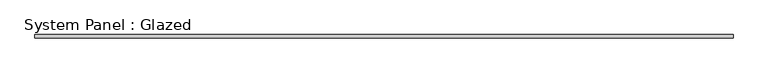
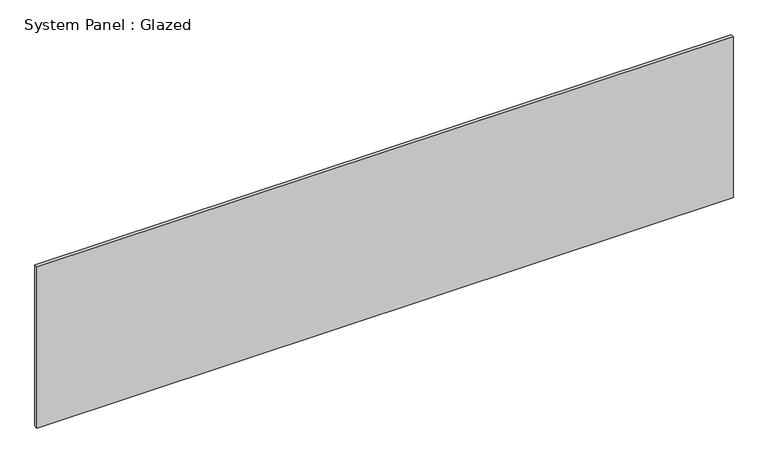
"""IFC4 building model written with IfcOpenShell, lengths in millimetres: plate geometry, System Panel : Glazed."""

from ifc_helpers import new_model, si_unit, origin, origin_with_axes, place, context, project, spatial, polyline, outline, extrude, source, transform, mapped, element, save


def system_panel_glazed_542b97c0(model_context):
    return source(origin(), model_context, "Body", "SweptSolid", [
        extrude(outline(polyline([(2492.375, 19.05), (-2492.375, 19.05), (-2492.375, 44.45), (2492.375, 44.45), (2492.375, 19.05)])), origin_with_axes(), (0.0, 0.0, 1.0), 1219.2),
    ])


if __name__ == "__main__":
    model = new_model("IFC4")
    model_context = context("Model", 3, world=origin())
    ifc_project = project(units=[si_unit("LENGTHUNIT", "METRE", prefix="MILLI")], contexts=[model_context])
    site = spatial("IfcSite", under=ifc_project)
    building = spatial("IfcBuilding", under=site)
    placement = place(None, origin())
    system_panel_glazed_shape = system_panel_glazed_542b97c0(model_context)
    element("IfcPlate", 1, ObjectType="System Panel : Glazed", at=placement, inside=building, context=model_context, shape_type="MappedRepresentation", body=[
        mapped(system_panel_glazed_shape, transform((0.0, 0.0, 0.0), x_axis=(1.0, 0.0, 0.0), y_axis=(0.0, 1.0, 0.0), z_axis=(0.0, 0.0, 1.0))),
    ])
    save(model, "model.ifc")

# Revit data of these elements
# Type "System Panel : Glazed"
#   Construction Type Id = "GSP4R"
#   Analytic Construction = "1/8 in Pilkington single glazing"
#   Visual Light Transmittance = 0.9
#   Solar Heat Gain Coefficient = 0.86
#   Heat Transfer Coefficient (U) = 1.18115 BTU/(h·ft²·°F)
# Element 1 (IfcPlate, "System Panel : Glazed")
#   Materials on its faces: "Glass"
# Materials
#   "Glass": class "Glass", colour RGB 0 128 192, transparency 0.75, Description = "Soda Lime Glass", Cost = 0
